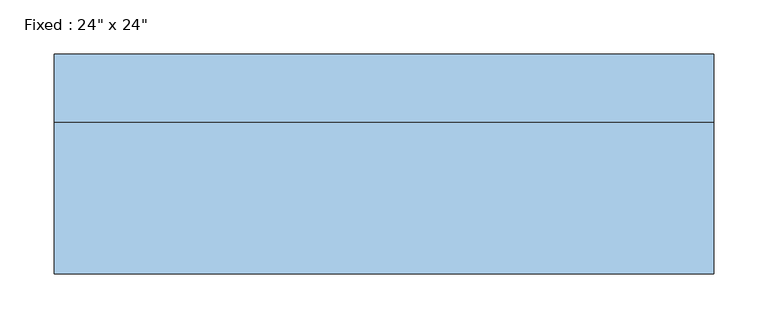
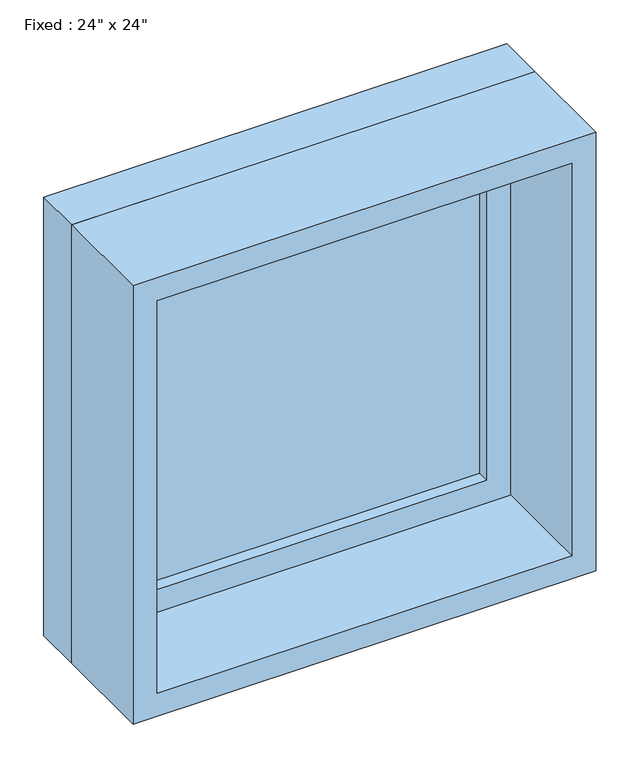
"""IFC4 building model written with IfcOpenShell, lengths in millimetres: window geometry."""

from ifc_helpers import new_model, si_unit, frame, origin, place, context, project, spatial, polyline, outline, extrude, source, transform, mapped, element, save


def window_6846e476(model_context):
    return source(origin(), model_context, "Body", "SweptSolid", [
        extrude(outline(polyline([(203.2, 53.975), (-279.4, 53.975), (-279.4, 66.675), (203.2, 66.675), (203.2, 53.975)])), frame((0.0, 0.0, 977.9), z_axis=(0.0, 0.0, 1.0), x_axis=(1.0, 0.0, 0.0)), (0.0, 0.0, 1.0), 482.6),
        extrude(outline(polyline([(1504.95, -323.85), (933.45, -323.85), (933.45, 247.65), (1504.95, 247.65), (1504.95, -323.85)]), holes=[polyline([(1460.5, -279.4), (1460.5, 203.2), (977.9, 203.2), (977.9, -279.4), (1460.5, -279.4)])]), frame((0.0, 38.1, 0.0), z_axis=(0.0, 1.0, 0.0), x_axis=(0.0, 0.0, 1.0)), (0.0, 0.0, 1.0), 44.45),
        extrude(outline(polyline([(1524.0, -342.9), (914.4, -342.9), (914.4, 266.7), (1524.0, 266.7), (1524.0, -342.9)]), holes=[polyline([(1492.25, -311.15), (1492.25, 234.95), (946.15, 234.95), (946.15, -311.15), (1492.25, -311.15)])]), frame((0.0, -101.6, 0.0), z_axis=(0.0, 1.0, 0.0), x_axis=(0.0, 0.0, 1.0)), (0.0, 0.0, 1.0), 139.7),
        extrude(outline(polyline([(1524.0, 266.7), (1524.0, -342.9), (914.4, -342.9), (914.4, 266.7), (1524.0, 266.7)]), holes=[polyline([(1504.95, 247.65), (933.45, 247.65), (933.45, -323.85), (1504.95, -323.85), (1504.95, 247.65)])]), frame((0.0, 38.1, 0.0), z_axis=(0.0, 1.0, 0.0), x_axis=(0.0, 0.0, 1.0)), (0.0, 0.0, 1.0), 63.5),
    ])


if __name__ == "__main__":
    model = new_model("IFC4")
    model_context = context("Model", 3, world=origin())
    ifc_project = project(units=[si_unit("LENGTHUNIT", "METRE", prefix="MILLI")], contexts=[model_context])
    site = spatial("IfcSite", under=ifc_project)
    building = spatial("IfcBuilding", under=site)
    placement = place(None, origin())
    window_shape = window_6846e476(model_context)
    element("IfcWindow", 1, ObjectType="Fixed : 24\" x 24\"", at=placement, inside=building, context=model_context, shape_type="MappedRepresentation", body=[
        mapped(window_shape, transform((0.0, 0.0, 0.0), x_axis=(1.0, 0.0, 0.0), y_axis=(0.0, 1.0, 0.0), z_axis=(0.0, 0.0, 1.0))),
    ])
    save(model, "model.ifc")

# Revit data of these elements
# Type "Fixed : 24\" x 24\""
#   Type Mark = "3"
#   Construction Type Id = "GSP4R"
#   Assembly Code = "B2020100"
#   Analytic Construction = "1/8 in Pilkington single glazing"
#   Visual Light Transmittance = 0.9
#   Solar Heat Gain Coefficient = 0.78
#   Heat Transfer Coefficient (U) = 0.6496 BTU/(h·ft²·°F)
#   Height = 2' - 0"
#   Default Sill Height = 3' - 0"
#   Width = 2' - 0"
#   Window Inset = 0' - 0 3/4"
#   Define Thermal Properties by = 1
#   Define Thermal Properties by = 1
#   Glass Pane Material = Glass
#   Sash Material = Sash
#   Wall Closure = (empty or 0)
# Element 1 (IfcWindow, "Fixed : 24\" x 24\"")
#   Materials on its faces: "Sash", "Glass"
# Materials
#   "Glass": class "Glass", colour RGB 0 128 192, transparency 0.75, Description = "Soda Lime Glass", Cost = 0
#   "Sash": class "Wood", colour RGB 224 178 126, transparency 0, Cost = 0
